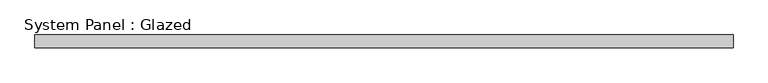
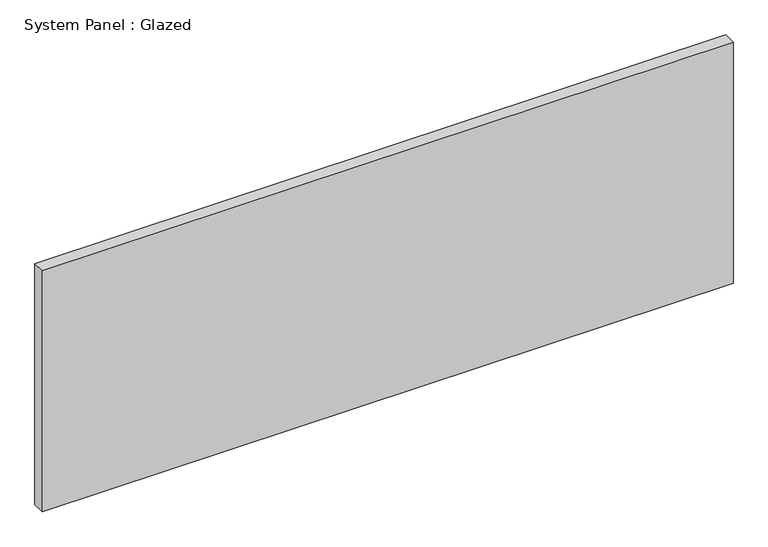
"""IFC4 building model written with IfcOpenShell, lengths in millimetres: plate geometry, System Panel : Glazed."""

from ifc_helpers import new_model, si_unit, origin, origin_with_axes, place, context, project, spatial, polyline, outline, extrude, source, transform, mapped, element, save


def system_panel_glazed_2f197d06(model_context):
    return source(origin(), model_context, "Body", "SweptSolid", [
        extrude(outline(polyline([(697.4416667, 19.05), (-697.4416667, 19.05), (-697.4416667, 44.45), (697.4416667, 44.45), (697.4416667, 19.05)])), origin_with_axes(), (0.0, 0.0, 1.0), 514.35),
    ])


if __name__ == "__main__":
    model = new_model("IFC4")
    model_context = context("Model", 3, world=origin())
    ifc_project = project(units=[si_unit("LENGTHUNIT", "METRE", prefix="MILLI")], contexts=[model_context])
    site = spatial("IfcSite", under=ifc_project)
    building = spatial("IfcBuilding", under=site)
    placement = place(None, origin())
    system_panel_glazed_shape = system_panel_glazed_2f197d06(model_context)
    element("IfcPlate", 1, ObjectType="System Panel : Glazed", at=placement, inside=building, context=model_context, shape_type="MappedRepresentation", body=[
        mapped(system_panel_glazed_shape, transform((0.0, 0.0, 0.0), x_axis=(1.0, 0.0, 0.0), y_axis=(0.0, 1.0, 0.0), z_axis=(0.0, 0.0, 1.0))),
    ])
    save(model, "model.ifc")

# Revit data of these elements
# Type "System Panel : Glazed"
#   Construction Type Id = "GSP4R"
#   Analytic Construction = "1/8 in Pilkington single glazing"
#   Visual Light Transmittance = 0.9
#   Solar Heat Gain Coefficient = 0.86
#   Heat Transfer Coefficient (U) = 1.18115 BTU/(h·ft²·°F)
# Element 1 (IfcPlate, "System Panel : Glazed")
#   Materials on its faces: "Glass"
# Materials
#   "Glass": class "Glass", colour RGB 0 128 192, transparency 0.75, Description = "Soda Lime Glass", Cost = 0
